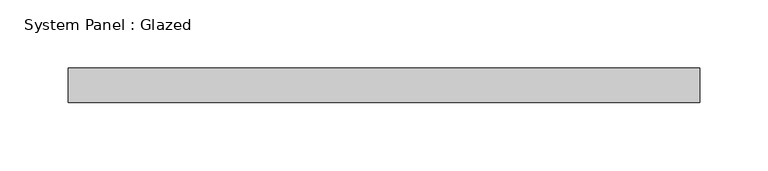
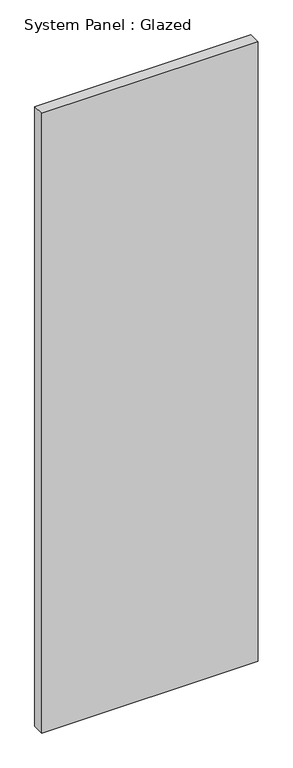
"""IFC4 building model written with IfcOpenShell, lengths in millimetres: plate geometry, System Panel : Glazed."""

from ifc_helpers import new_model, si_unit, origin, origin_with_axes, place, context, project, spatial, polyline, outline, extrude, source, transform, mapped, element, save


def system_panel_glazed_7c06924b(model_context):
    return source(origin(), model_context, "Body", "SweptSolid", [
        extrude(outline(polyline([(231.775, 19.05), (-231.775, 19.05), (-231.775, 44.45), (231.775, 44.45), (231.775, 19.05)])), origin_with_axes(), (0.0, 0.0, 1.0), 1402.3594037),
    ])


if __name__ == "__main__":
    model = new_model("IFC4")
    model_context = context("Model", 3, world=origin())
    ifc_project = project(units=[si_unit("LENGTHUNIT", "METRE", prefix="MILLI")], contexts=[model_context])
    site = spatial("IfcSite", under=ifc_project)
    building = spatial("IfcBuilding", under=site)
    placement = place(None, origin())
    system_panel_glazed_shape = system_panel_glazed_7c06924b(model_context)
    element("IfcPlate", 1, ObjectType="System Panel : Glazed", at=placement, inside=building, context=model_context, shape_type="MappedRepresentation", body=[
        mapped(system_panel_glazed_shape, transform((0.0, 0.0, 0.0), x_axis=(1.0, 0.0, 0.0), y_axis=(0.0, 1.0, 0.0), z_axis=(0.0, 0.0, 1.0))),
    ])
    save(model, "model.ifc")

# Revit data of these elements
# Type "System Panel : Glazed"
#   Construction Type Id = "GSP4R"
#   Analytic Construction = "1/8 in Pilkington single glazing"
#   Visual Light Transmittance = 0.9
#   Solar Heat Gain Coefficient = 0.86
#   Heat Transfer Coefficient (U) = 1.18115 BTU/(h·ft²·°F)
#   Define Thermal Properties by = 1
# Element 1 (IfcPlate, "System Panel : Glazed")
#   Materials on its faces: "Glass"
# Materials
#   "Glass": class "Glass", colour RGB 0 128 192, transparency 0.75, Description = "Soda Lime Glass", Cost = 0
